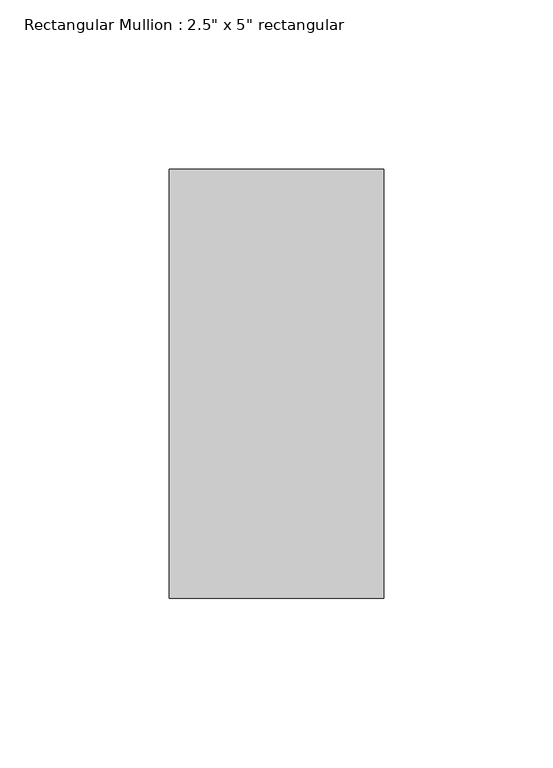
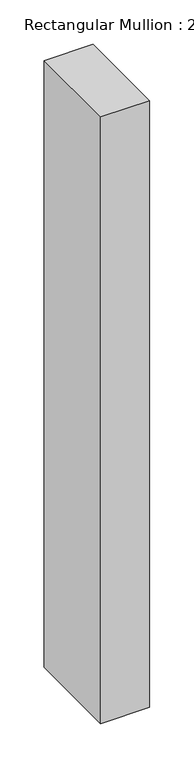
"""IFC4 building model written with IfcOpenShell, lengths in millimetres: member geometry."""

from ifc_helpers import new_model, si_unit, frame, origin, place, context, project, spatial, polyline, outline, extrude, source, transform, mapped, element, save


def member_5ab2641c(model_context):
    return source(origin(), model_context, "Body", "SweptSolid", [
        extrude(outline(polyline([(31.75, 63.5), (31.75, -63.5), (-31.75, -63.5), (-31.75, 63.5), (31.75, 63.5)])), frame((0.0, 0.0, -832.5361093), z_axis=(0.0, 0.0, 1.0), x_axis=(1.0, 0.0, 0.0)), (0.0, 0.0, 1.0), 832.5361093),
    ])


if __name__ == "__main__":
    model = new_model("IFC4")
    model_context = context("Model", 3, world=origin())
    ifc_project = project(units=[si_unit("LENGTHUNIT", "METRE", prefix="MILLI")], contexts=[model_context])
    site = spatial("IfcSite", under=ifc_project)
    building = spatial("IfcBuilding", under=site)
    placement = place(None, origin())
    member_shape = member_5ab2641c(model_context)
    element("IfcMember", 1, ObjectType="Rectangular Mullion : 2.5\" x 5\" rectangular", at=placement, inside=building, context=model_context, shape_type="MappedRepresentation", body=[
        mapped(member_shape, transform((0.0, 0.0, 0.0), x_axis=(1.0, 0.0, 0.0), y_axis=(0.0, 1.0, 0.0), z_axis=(0.0, 0.0, 1.0))),
    ])
    save(model, "model.ifc")

# Revit data of these elements
# Type "Rectangular Mullion : 2.5\" x 5\" rectangular"
#   built-in parameter 1007304 = 0.416667 (stored number, unit not read)
#   built-in parameter 1007301 = 0.104167 (stored number, unit not read)
#   built-in parameter 1007300 = 0.104167 (stored number, unit not read)
# Element 1 (IfcMember, "Rectangular Mullion : 2.5\" x 5\" rectangular")
#   Materials on its faces: "Aluminum"
# Materials
#   "Aluminum": class "Metal", colour RGB 247 247 247, transparency 0, Description = "Aluminum 6061", Cost = 0
